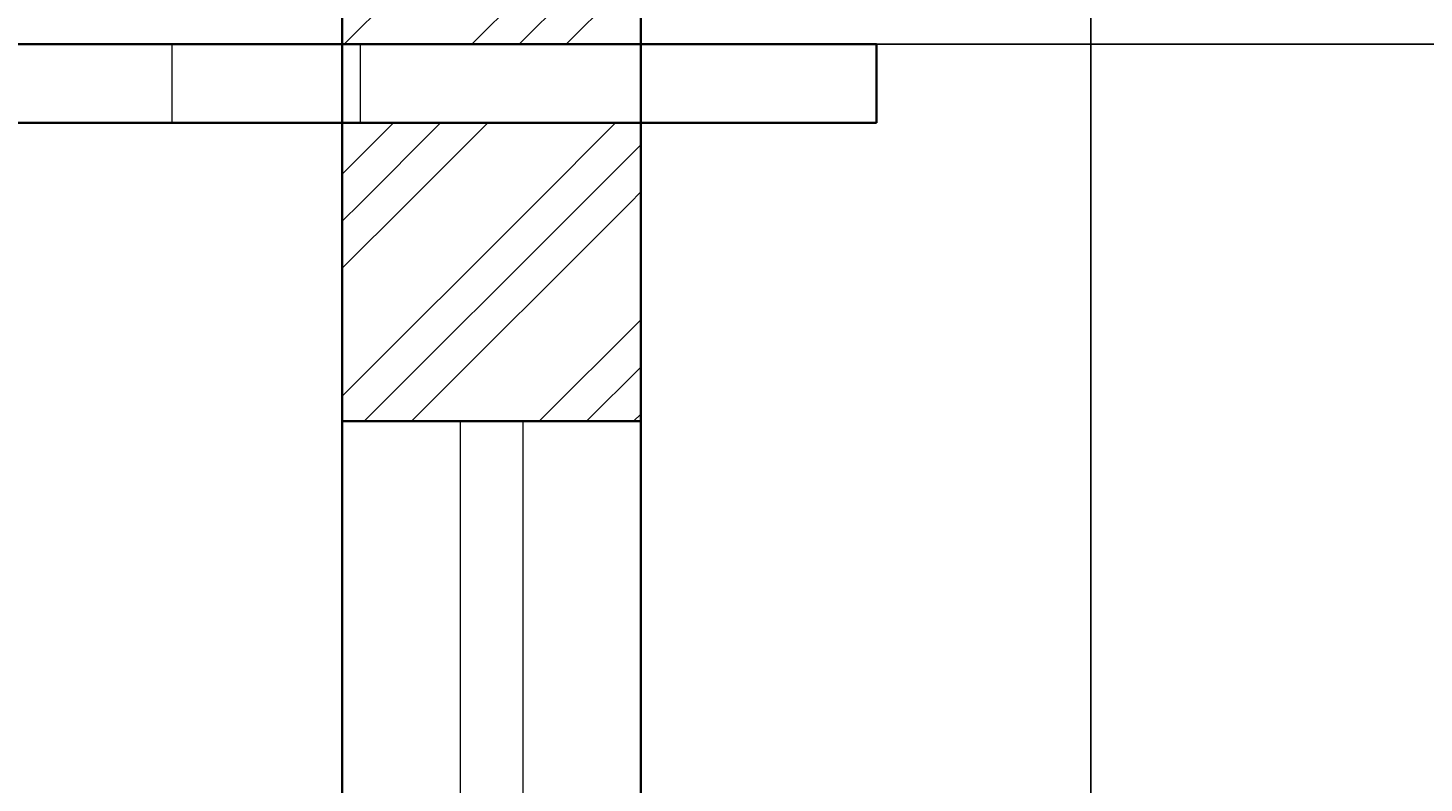
# Model space of a CAD drawing. Units: inches. Extents: x -128 to 854, y -395 to 398.
# Tile 19 of 61: x 279 to 368, y -249 to -201. Entities that reach past the tile are written whole.
import ezdxf

# ---------------------------------------------------------------- set-up
doc = ezdxf.new("R2010")
doc.units = ezdxf.units.IN
doc.header["$MEASUREMENT"] = 0
for name, color, linetype, lineweight in [('A-ANNO-DIMS', 2, 'Continuous', 18), ('A-GLAZ', 220, 'Continuous', 18), ('A-SECT', 220, 'Continuous', 35), ('A-SECT-PATT', 8, 'Continuous', 13)]:
    doc.layers.add(name, color=color, linetype=linetype, lineweight=lineweight)
doc.styles.get("Standard").update_dxf_attribs({"font": 'arial.ttf'})
doc.dimstyles.get("Standard").update_dxf_attribs({"dimtxt": 0.18, "dimasz": 0.18, "dimexe": 0.18, "dimexo": 0.0625, "dimgap": 0.09, "dimtad": 0, "dimtih": 1, "dimtoh": 1, "dimdec": 1, "dimzin": 0, "dimdsep": 46, "dimlunit": 4, "dimtxsty": 'Standard', "dimcen": 0.09, "dimclrd": 1, "dimclre": 2, "dimclrt": 6, "dimadec": 0, "dimazin": 0, "dimtfac": 1, "dimtdec": 1, "dimtofl": 0, "dimtmove": 0, "dimatfit": 3, "dimfxl": 1, "dimtfill": 2, "dimtfillclr": 3, "dimtolj": 1, "dimtzin": 0, "dimarcsym": 0})

# ---------------------------------------------------------------- blocks, each defined once
blk = doc.blocks.new('*D120')
at = {"layer": 'A-ANNO-DIMS', "color": 2, "lineweight": -2, "transparency": 16777216}
for p, q in [((317.902, -178.019), (389.719, -178.019)), ((337.902, -358.019), (389.719, -358.019))]:
    blk.add_line(p, q, dxfattribs=at)
at = {"layer": 'A-ANNO-DIMS', "color": 1, "lineweight": -2, "transparency": 16777216}
for p, q in [((389.539, -178.199), (389.539, -267.837)), ((389.539, -357.839), (389.539, -268.201))]:
    blk.add_line(p, q, dxfattribs=at)
at = {"layer": 'A-ANNO-DIMS', "color": 1, "transparency": 16777216}
for points in [[(389.509, -178.199), (389.569, -178.199), (389.539, -178.019)], [(389.509, -357.839), (389.569, -357.839), (389.539, -358.019)]]:
    blk.add_solid(points, dxfattribs=at)
at = {"layer": 'Defpoints', "color": 0, "transparency": 16777216}
for p in [(317.839, -178.019), (337.839, -358.019), (389.539, -358.019)]:
    blk.add_point(p, dxfattribs=at)
at = {"layer": 'A-ANNO-DIMS', "color": 6, "transparency": 16777216, "insert": (389.539, -268.019), "char_height": 0.18, "attachment_point": 5, "bg_fill": 1, "box_fill_scale": 1.25, "bg_fill_color": 3, "bg_fill_transparency": 0}
blk.add_mtext('\\A1;15\'-0"', dxfattribs=at)
blk = doc.blocks.new('*D127')
at = {"layer": 'A-ANNO-DIMS', "color": 2, "lineweight": -2, "transparency": 16777216}
for p, q in [((260.902, -202.019), (389.719, -202.019)), ((317.902, -298.019), (389.719, -298.019))]:
    blk.add_line(p, q, dxfattribs=at)
at = {"layer": 'A-ANNO-DIMS', "color": 1, "lineweight": -2, "transparency": 16777216}
for p, q in [((389.539, -202.199), (389.539, -249.837)), ((389.539, -297.839), (389.539, -250.201))]:
    blk.add_line(p, q, dxfattribs=at)
at = {"layer": 'A-ANNO-DIMS', "color": 1, "transparency": 16777216}
for points in [[(389.509, -202.199), (389.569, -202.199), (389.539, -202.019)], [(389.509, -297.839), (389.569, -297.839), (389.539, -298.019)]]:
    blk.add_solid(points, dxfattribs=at)
at = {"layer": 'Defpoints', "color": 0, "transparency": 16777216}
for p in [(260.839, -202.019), (389.539, -202.019), (317.839, -298.019)]:
    blk.add_point(p, dxfattribs=at)
at = {"layer": 'A-ANNO-DIMS', "color": 6, "transparency": 16777216, "insert": (389.539, -250.019), "char_height": 0.18, "attachment_point": 5, "bg_fill": 1, "box_fill_scale": 1.25, "bg_fill_color": 3, "bg_fill_transparency": 0}
blk.add_mtext('\\A1;8\'-0"', dxfattribs=at)
blk = doc.blocks.new('*D134')
at = {"layer": 'A-ANNO-DIMS', "color": 2, "lineweight": -2, "transparency": 16777216}
for p, q in [((418.217, -191.476), (346.3, -191.476)), ((418.217, -371.476), (346.3, -371.476))]:
    blk.add_line(p, q, dxfattribs=at)
at = {"layer": 'A-ANNO-DIMS', "color": 1, "lineweight": -2, "transparency": 16777216}
for p, q in [((346.48, -191.656), (346.48, -281.295)), ((346.48, -371.296), (346.48, -281.658))]:
    blk.add_line(p, q, dxfattribs=at)
at = {"layer": 'A-ANNO-DIMS', "color": 1, "transparency": 16777216}
for points in [[(346.45, -191.656), (346.51, -191.656), (346.48, -191.476)], [(346.45, -371.296), (346.51, -371.296), (346.48, -371.476)]]:
    blk.add_solid(points, dxfattribs=at)
at = {"layer": 'Defpoints', "color": 0, "transparency": 16777216}
for p in [(346.48, -191.476), (418.28, -191.476), (418.28, -371.476)]:
    blk.add_point(p, dxfattribs=at)
at = {"layer": 'A-ANNO-DIMS', "color": 6, "transparency": 16777216, "insert": (346.48, -281.476), "char_height": 0.18, "attachment_point": 5, "bg_fill": 1, "box_fill_scale": 1.25, "bg_fill_color": 3, "bg_fill_transparency": 0}
blk.add_mtext('\\A1;15\'-0"', dxfattribs=at)

msp = doc.modelspace()

# ---------------------------------------------------------------- hatches: boundary and pattern name
at = {"layer": 'A-SECT-PATT'}
h = msp.add_hatch(dxfattribs=at)
h.set_pattern_fill('GOST_GROUND', color=256)
h.set_pattern_definition([(45, (0, 0), (14.14214, -9e-16), [20]), (45, (3, 0), (14.14214, -9e-16), [20]), (45, (6, 0), (14.14214, -9e-16), [20])])
h.paths.add_polyline_path([(-37.161, -178.019), (-56.161, -178.019), (-56.161, -202.019), (-37.161, -202.019)])
h.paths.add_polyline_path([(160.839, -178.019), (141.839, -178.019), (141.839, -202.019), (160.839, -202.019)])
h.paths.add_polyline_path([(160.839, -207.019), (141.839, -207.019), (141.839, -226.019), (160.839, -226.019)])
h.paths.add_polyline_path([(317.839, -178.019), (298.839, -178.019), (298.839, -202.019), (317.839, -202.019)])
h.paths.add_polyline_path([(317.839, -207.019), (298.839, -207.019), (298.839, -226.019), (317.839, -226.019)])
h.paths.add_polyline_path([(317.839, -274.019), (298.839, -274.019), (298.839, -298.019), (303.839, -298.019), (312.839, -298.019), (317.839, -298.019)])
h = msp.add_hatch(dxfattribs=at)
h.set_pattern_fill('ANSI31', color=256, scale=96, angle=45, style=0)
h.paths.add_polyline_path([(-38.361, -202.019), (300.039, -202.019), (300.039, -207.019), (-38.361, -207.019)])

# ---------------------------------------------------------------- linework, layer by layer
at = {"layer": 'A-GLAZ'}
for p, q in [((306.339, -226.019), (306.339, -274.019)), ((310.339, -226.019), (310.339, -274.019))]:
    msp.add_line(p, q, dxfattribs=at)
at = {"layer": 'A-SECT'}
for p, q in [((298.839, -298.019), (298.839, -178.019)), ((317.839, -298.019), (317.839, -178.019)), ((-56.161, -202.019), (317.839, -202.019)), ((317.839, -202.019), (327.839, -202.019)), ((327.839, -202.019), (332.839, -202.019)), ((332.839, -202.019), (332.839, -207.019)), ((-56.161, -207.019), (317.839, -207.019)), ((332.839, -207.019), (317.839, -207.019)), ((298.839, -226.019), (317.839, -226.019))]:
    msp.add_line(p, q, dxfattribs=at)

# ---------------------------------------------------------------- dimensions: what is measured, and where the dimension line sits
at = {"layer": 'A-ANNO-DIMS'}
for base, p1, p2, picture, middle in [((389.539, -358.019), (317.839, -178.019), (337.839, -358.019), '*D120', (389.539, -268.019)), ((346.48, -191.476), (418.28, -371.476), (418.28, -191.476), '*D134', (346.48, -281.476)), ((389.539, -202.019), (317.839, -298.019), (260.839, -202.019), '*D127', (389.539, -250.019))]:
    dim = msp.add_linear_dim(base=base, p1=p1, p2=p2, angle=90, dimstyle='Standard', override={"dimdec": 1, "dimlfac": 1, "dimrnd": 0, "dimzin": 1, "dimdsep": 46, "dimlunit": 4, "dimfrac": 2}, dxfattribs=at)
    dim.commit()
    dim.dimension.update_dxf_attribs({"geometry": picture, "text_midpoint": middle})

doc.saveas('drawing.dxf')
